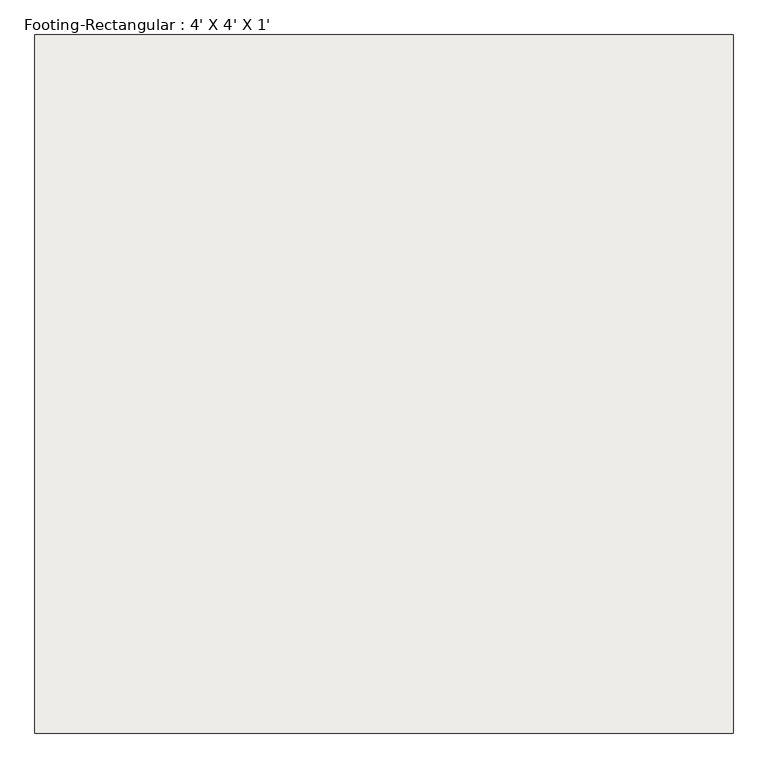
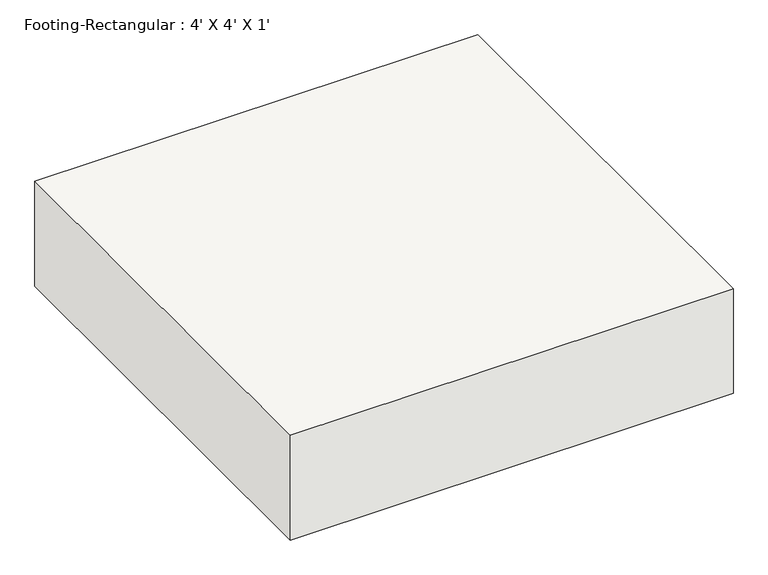
"""IFC4 building model written with IfcOpenShell, lengths in millimetres: slab geometry, Footing-Rectangular : 4' X 4' X 1'."""

from ifc_helpers import new_model, si_unit, frame, origin, place, context, project, spatial, polyline, outline, extrude, source, transform, mapped, element, save


def footing_rectangular_4_x_4_x_1_cc6aa31b(model_context):
    return source(origin(), model_context, "Body", "SweptSolid", [
        extrude(outline(polyline([(609.6, 609.6), (609.6, -609.6), (-609.6, -609.6), (-609.6, 609.6), (609.6, 609.6)])), frame((0.0, 0.0, -304.8), z_axis=(0.0, 0.0, 1.0), x_axis=(1.0, 0.0, 0.0)), (0.0, 0.0, 1.0), 304.8),
    ])


if __name__ == "__main__":
    model = new_model("IFC4")
    model_context = context("Model", 3, world=origin())
    ifc_project = project(units=[si_unit("LENGTHUNIT", "METRE", prefix="MILLI")], contexts=[model_context])
    site = spatial("IfcSite", under=ifc_project)
    building = spatial("IfcBuilding", under=site)
    placement = place(None, origin())
    footing_rectangular_4_x_4_x_1_shape = footing_rectangular_4_x_4_x_1_cc6aa31b(model_context)
    element("IfcSlab", 1, ObjectType="Footing-Rectangular : 4' X 4' X 1'", at=placement, inside=building, context=model_context, shape_type="MappedRepresentation", body=[
        mapped(footing_rectangular_4_x_4_x_1_shape, transform((0.0, 0.0, 0.0), x_axis=(1.0, 0.0, 0.0), y_axis=(0.0, 1.0, 0.0), z_axis=(0.0, 0.0, 1.0))),
    ])
    save(model, "model.ifc")

# Revit data of these elements
# Type "Footing-Rectangular : 4' X 4' X 1'"
#   Assembly Code = "A1010100"
#   Width = 4' - 0"
#   Length = 4' - 0"
#   Foundation Thickness = 1' - 0"
#   Structural Material [instance default] = Concrete, Cast-in-Place gray
# Element 1 (IfcSlab, "Footing-Rectangular : 4' X 4' X 1'")
#   Materials on its faces: "Concrete, Cast-in-Place gray"
# Materials
#   "Concrete, Cast-in-Place gray": class "Concrete", colour RGB 192 192 192, transparency 0, Description = "Cast-in-place concrete", Cost = 0
